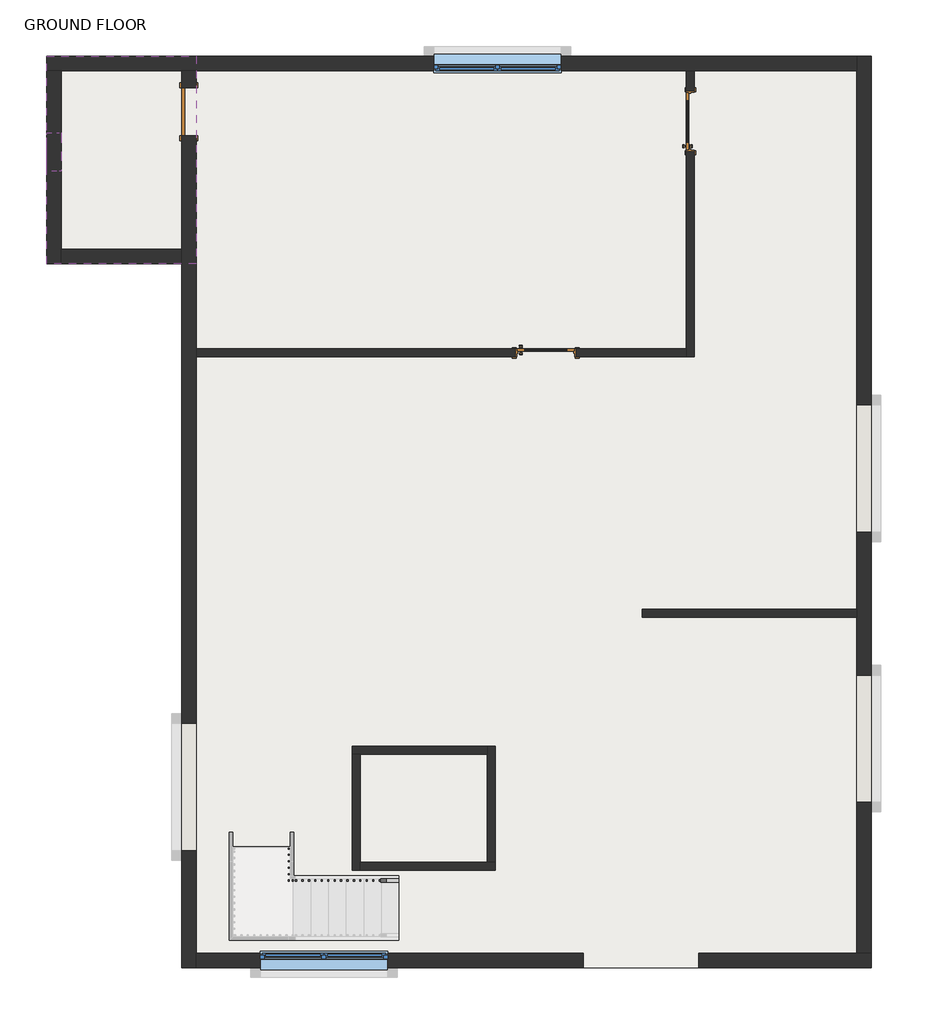
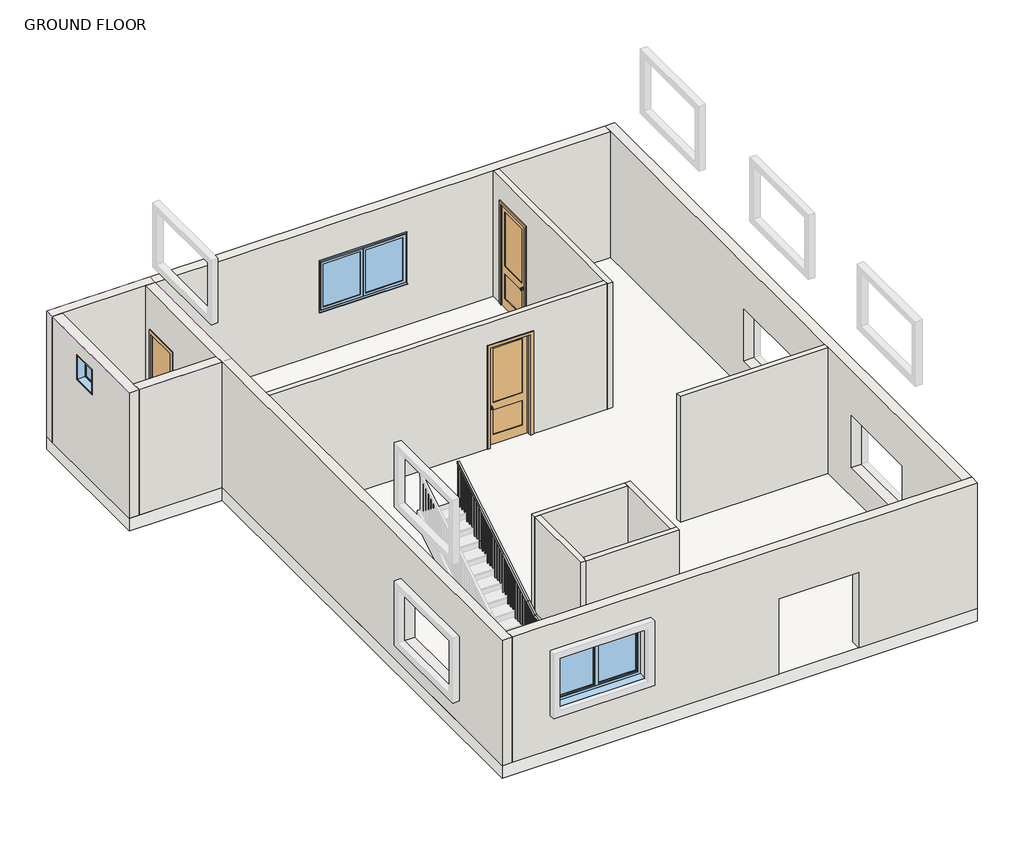
# One storey, part 1 of 2: 13 walls, 3 doors, 3 windows, 1 railing, 1 roof, 1 slab.
"""IFC4 building model written with IfcOpenShell, lengths in millimetres."""

from ifc_helpers import new_model, si_unit, frame, origin, origin_with_axes, place, context, project, spatial, polyline, outline, extrude, faceted_brep, transform, mapped, element, save
from components import door_1a517266, door_a1484949, window_80340324, w2_w2_7b90d420

model = new_model("IFC4")

# Units and contexts
model_context = context("Model", 3, world=origin())
ifc_project = project(units=[si_unit("LENGTHUNIT", "METRE", prefix="MILLI")], contexts=[model_context])

# Site, building, storey
site = spatial("IfcSite", under=ifc_project)
building = spatial("IfcBuilding", under=site)
storey = spatial("IfcBuildingStorey", under=building, Name="GROUND FLOOR", Elevation=304.8)

# Doors
placement = place(None, origin())
door_shape = door_1a517266(model_context)
element("IfcDoor", 1, ObjectType="Door-Interior-Single-2_Panel-Wood : 36\" x 96\"", at=placement, inside=storey, context=model_context, shape_type="MappedRepresentation", body=[
    mapped(door_shape, transform((-1003.5474631, 5446.3811648, 304.8), x_axis=(1.0, 0.0, 0.0), y_axis=(0.0, 1.0, 0.0), z_axis=(0.0, 0.0, 1.0))),
])
element("IfcDoor", 2, ObjectType="Door-Interior-Single-2_Panel-Wood : 36\" x 96\"", at=placement, inside=storey, context=model_context, shape_type="MappedRepresentation", body=[
    mapped(door_shape, transform((1279.2775369, 9100.8061648, 304.8), x_axis=(0.0, 1.0, 0.0), y_axis=(-1.0, 0.0, 0.0), z_axis=(0.0, 0.0, 1.0))),
])
door_2_shape = door_a1484949(model_context)
element("IfcDoor", 3, ObjectType="Single-Flush : 30\" x 80\"", at=placement, inside=storey, context=model_context, shape_type="MappedRepresentation", body=[
    mapped(door_2_shape, transform((-6642.3474631, 9253.2061648, 304.8), x_axis=(0.0, 1.0, 0.0), y_axis=(-1.0, 0.0, 0.0), z_axis=(0.0, 0.0, 1.0))),
])

# Railing
element("IfcRailing", 4, ObjectType="Handrail - Rectangular", at=placement, inside=storey, context=model_context, shape_type="SolidModel", body=[
    faceted_brep([(-3322.4601025, -2919.857314, 1388.5333333), (-3322.4601025, -2919.857314, 1329.1318731), (-3322.4601025, -2869.057314, 1329.1318731), (-3322.4601025, -2869.057314, 1388.5333333), (-4998.8601025, -2919.857314, 2404.5333333), (-5013.0525119, -2919.857314, 2353.7333333), (-5013.0525119, -2869.057314, 2353.7333333), (-4998.8601025, -2869.057314, 2404.5333333), (-5087.9750936, -2919.857314, 2404.5333333), (-5087.9750936, -2919.857314, 2353.7333333), (-5037.1750936, -2869.057314, 2353.7333333), (-5037.1750936, -2869.057314, 2404.5333333), (-5087.9750936, -2670.5272484, 2404.5333333), (-5087.9750936, -2656.334839, 2353.7333333), (-5037.1750936, -2656.334839, 2353.7333333), (-5037.1750936, -2670.5272484, 2404.5333333), (-5087.9750936, -2391.1272484, 2573.8666667), (-5087.9750936, -2364.7975213, 2530.4226168), (-5037.1750936, -2364.7975213, 2530.4226168), (-5037.1750936, -2391.1272484, 2573.8666667), (-5087.9750936, 402.8727516, 4267.2), (-5037.1750936, 402.8727516, 4267.2), (-5037.1750936, 402.8727516, 4207.7985397), (-5087.9750936, 402.8727516, 4207.7985397)], [[[0, 1, 2, 3]], [[1, 0, 4, 5]], [[2, 1, 5, 6]], [[3, 2, 6, 7]], [[0, 3, 7, 4]], [[5, 4, 8, 9]], [[6, 5, 9, 10]], [[7, 6, 10, 11]], [[4, 7, 11, 8]], [[9, 8, 12, 13]], [[10, 9, 13, 14]], [[11, 10, 14, 15]], [[8, 11, 15, 12]], [[13, 12, 16, 17]], [[14, 13, 17, 18]], [[15, 14, 18, 19]], [[12, 15, 19, 16]], [[20, 21, 22, 23]], [[17, 16, 20, 23]], [[18, 17, 23, 22]], [[19, 18, 22, 21]], [[16, 19, 21, 20]]]),
    extrude(outline(polyline([(342.5477516, 4171.2379337), (361.5977516, 4182.7833882), (361.5977516, 3183.4666667), (342.5477516, 3183.4666667), (342.5477516, 4171.2379337)])), frame((-5072.1000936, 0.0, 0.0), z_axis=(1.0, 0.0, 0.0), x_axis=(0.0, 1.0, 0.0)), (0.0, 0.0, 1.0), 19.05),
    extrude(outline(polyline([(240.9477516, 4109.6621761), (259.9977516, 4121.2076307), (259.9977516, 3183.4666667), (240.9477516, 3183.4666667), (240.9477516, 4109.6621761)])), frame((-5072.1000936, 0.0, 0.0), z_axis=(1.0, 0.0, 0.0), x_axis=(0.0, 1.0, 0.0)), (0.0, 0.0, 1.0), 19.05),
    extrude(outline(polyline([(139.3477516, 4048.0864185), (158.3977516, 4059.6318731), (158.3977516, 3183.4666667), (139.3477516, 3183.4666667), (139.3477516, 4048.0864185)])), frame((-5072.1000936, 0.0, 0.0), z_axis=(1.0, 0.0, 0.0), x_axis=(0.0, 1.0, 0.0)), (0.0, 0.0, 1.0), 19.05),
    extrude(outline(polyline([(37.7477516, 3986.510661), (56.7977516, 3998.0561155), (56.7977516, 3014.1333333), (37.7477516, 3014.1333333), (37.7477516, 3986.510661)])), frame((-5072.1000936, 0.0, 0.0), z_axis=(1.0, 0.0, 0.0), x_axis=(0.0, 1.0, 0.0)), (0.0, 0.0, 1.0), 19.05),
    extrude(outline(polyline([(-63.8522484, 3924.9349034), (-44.8022484, 3936.4803579), (-44.8022484, 3014.1333333), (-63.8522484, 3014.1333333), (-63.8522484, 3924.9349034)])), frame((-5072.1000936, 0.0, 0.0), z_axis=(1.0, 0.0, 0.0), x_axis=(0.0, 1.0, 0.0)), (0.0, 0.0, 1.0), 19.05),
    extrude(outline(polyline([(-165.4522484, 3863.3591458), (-146.4022484, 3874.9046004), (-146.4022484, 3014.1333333), (-165.4522484, 3014.1333333), (-165.4522484, 3863.3591458)])), frame((-5072.1000936, 0.0, 0.0), z_axis=(1.0, 0.0, 0.0), x_axis=(0.0, 1.0, 0.0)), (0.0, 0.0, 1.0), 19.05),
    extrude(outline(polyline([(-267.0522484, 3801.7833882), (-248.0022484, 3813.3288428), (-248.0022484, 2844.8), (-267.0522484, 2844.8), (-267.0522484, 3801.7833882)])), frame((-5072.1000936, 0.0, 0.0), z_axis=(1.0, 0.0, 0.0), x_axis=(0.0, 1.0, 0.0)), (0.0, 0.0, 1.0), 19.05),
    extrude(outline(polyline([(-368.6522484, 3740.2076307), (-349.6022484, 3751.7530852), (-349.6022484, 2844.8), (-368.6522484, 2844.8), (-368.6522484, 3740.2076307)])), frame((-5072.1000936, 0.0, 0.0), z_axis=(1.0, 0.0, 0.0), x_axis=(0.0, 1.0, 0.0)), (0.0, 0.0, 1.0), 19.05),
    extrude(outline(polyline([(-470.2522484, 3678.6318731), (-451.2022484, 3690.1773276), (-451.2022484, 2675.4666667), (-470.2522484, 2675.4666667), (-470.2522484, 3678.6318731)])), frame((-5072.1000936, 0.0, 0.0), z_axis=(1.0, 0.0, 0.0), x_axis=(0.0, 1.0, 0.0)), (0.0, 0.0, 1.0), 19.05),
    extrude(outline(polyline([(-571.8522484, 3617.0561155), (-552.8022484, 3628.60157), (-552.8022484, 2675.4666667), (-571.8522484, 2675.4666667), (-571.8522484, 3617.0561155)])), frame((-5072.1000936, 0.0, 0.0), z_axis=(1.0, 0.0, 0.0), x_axis=(0.0, 1.0, 0.0)), (0.0, 0.0, 1.0), 19.05),
    extrude(outline(polyline([(-673.4522484, 3555.4803579), (-654.4022484, 3567.0258125), (-654.4022484, 2675.4666667), (-673.4522484, 2675.4666667), (-673.4522484, 3555.4803579)])), frame((-5072.1000936, 0.0, 0.0), z_axis=(1.0, 0.0, 0.0), x_axis=(0.0, 1.0, 0.0)), (0.0, 0.0, 1.0), 19.05),
    extrude(outline(polyline([(-775.0522484, 3493.9046004), (-756.0022484, 3505.4500549), (-756.0022484, 2506.1333333), (-775.0522484, 2506.1333333), (-775.0522484, 3493.9046004)])), frame((-5072.1000936, 0.0, 0.0), z_axis=(1.0, 0.0, 0.0), x_axis=(0.0, 1.0, 0.0)), (0.0, 0.0, 1.0), 19.05),
    extrude(outline(polyline([(-876.6522484, 3432.3288428), (-857.6022484, 3443.8742973), (-857.6022484, 2506.1333333), (-876.6522484, 2506.1333333), (-876.6522484, 3432.3288428)])), frame((-5072.1000936, 0.0, 0.0), z_axis=(1.0, 0.0, 0.0), x_axis=(0.0, 1.0, 0.0)), (0.0, 0.0, 1.0), 19.05),
    extrude(outline(polyline([(-978.2522484, 3370.7530852), (-959.2022484, 3382.2985397), (-959.2022484, 2506.1333333), (-978.2522484, 2506.1333333), (-978.2522484, 3370.7530852)])), frame((-5072.1000936, 0.0, 0.0), z_axis=(1.0, 0.0, 0.0), x_axis=(0.0, 1.0, 0.0)), (0.0, 0.0, 1.0), 19.05),
    extrude(outline(polyline([(-1079.8522484, 3309.1773276), (-1060.8022484, 3320.7227822), (-1060.8022484, 2336.8), (-1079.8522484, 2336.8), (-1079.8522484, 3309.1773276)])), frame((-5072.1000936, 0.0, 0.0), z_axis=(1.0, 0.0, 0.0), x_axis=(0.0, 1.0, 0.0)), (0.0, 0.0, 1.0), 19.05),
    extrude(outline(polyline([(-1181.4522484, 3247.60157), (-1162.4022484, 3259.1470246), (-1162.4022484, 2336.8), (-1181.4522484, 2336.8), (-1181.4522484, 3247.60157)])), frame((-5072.1000936, 0.0, 0.0), z_axis=(1.0, 0.0, 0.0), x_axis=(0.0, 1.0, 0.0)), (0.0, 0.0, 1.0), 19.05),
    extrude(outline(polyline([(-1283.0522484, 3186.0258125), (-1264.0022484, 3197.571267), (-1264.0022484, 2336.8), (-1283.0522484, 2336.8), (-1283.0522484, 3186.0258125)])), frame((-5072.1000936, 0.0, 0.0), z_axis=(1.0, 0.0, 0.0), x_axis=(0.0, 1.0, 0.0)), (0.0, 0.0, 1.0), 19.05),
    extrude(outline(polyline([(-1384.6522484, 3124.4500549), (-1365.6022484, 3135.9955094), (-1365.6022484, 2167.4666667), (-1384.6522484, 2167.4666667), (-1384.6522484, 3124.4500549)])), frame((-5072.1000936, 0.0, 0.0), z_axis=(1.0, 0.0, 0.0), x_axis=(0.0, 1.0, 0.0)), (0.0, 0.0, 1.0), 19.05),
    extrude(outline(polyline([(-1486.2522484, 3062.8742973), (-1467.2022484, 3074.4197519), (-1467.2022484, 2167.4666667), (-1486.2522484, 2167.4666667), (-1486.2522484, 3062.8742973)])), frame((-5072.1000936, 0.0, 0.0), z_axis=(1.0, 0.0, 0.0), x_axis=(0.0, 1.0, 0.0)), (0.0, 0.0, 1.0), 19.05),
    extrude(outline(polyline([(-1587.8522484, 3001.2985397), (-1568.8022484, 3012.8439943), (-1568.8022484, 1998.1333333), (-1587.8522484, 1998.1333333), (-1587.8522484, 3001.2985397)])), frame((-5072.1000936, 0.0, 0.0), z_axis=(1.0, 0.0, 0.0), x_axis=(0.0, 1.0, 0.0)), (0.0, 0.0, 1.0), 19.05),
    extrude(outline(polyline([(-1689.4522484, 2939.7227822), (-1670.4022484, 2951.2682367), (-1670.4022484, 1998.1333333), (-1689.4522484, 1998.1333333), (-1689.4522484, 2939.7227822)])), frame((-5072.1000936, 0.0, 0.0), z_axis=(1.0, 0.0, 0.0), x_axis=(0.0, 1.0, 0.0)), (0.0, 0.0, 1.0), 19.05),
    extrude(outline(polyline([(-1791.0522484, 2878.1470246), (-1772.0022484, 2889.6924791), (-1772.0022484, 1998.1333333), (-1791.0522484, 1998.1333333), (-1791.0522484, 2878.1470246)])), frame((-5072.1000936, 0.0, 0.0), z_axis=(1.0, 0.0, 0.0), x_axis=(0.0, 1.0, 0.0)), (0.0, 0.0, 1.0), 19.05),
    extrude(outline(polyline([(-1892.6522484, 2816.571267), (-1873.6022484, 2828.1167216), (-1873.6022484, 1828.8), (-1892.6522484, 1828.8), (-1892.6522484, 2816.571267)])), frame((-5072.1000936, 0.0, 0.0), z_axis=(1.0, 0.0, 0.0), x_axis=(0.0, 1.0, 0.0)), (0.0, 0.0, 1.0), 19.05),
    extrude(outline(polyline([(-1994.2522484, 2754.9955094), (-1975.2022484, 2766.540964), (-1975.2022484, 1828.8), (-1994.2522484, 1828.8), (-1994.2522484, 2754.9955094)])), frame((-5072.1000936, 0.0, 0.0), z_axis=(1.0, 0.0, 0.0), x_axis=(0.0, 1.0, 0.0)), (0.0, 0.0, 1.0), 19.05),
    extrude(outline(polyline([(-2095.8522484, 2693.4197519), (-2076.8022484, 2704.9652064), (-2076.8022484, 1828.8), (-2095.8522484, 1828.8), (-2095.8522484, 2693.4197519)])), frame((-5072.1000936, 0.0, 0.0), z_axis=(1.0, 0.0, 0.0), x_axis=(0.0, 1.0, 0.0)), (0.0, 0.0, 1.0), 19.05),
    extrude(outline(polyline([(-2197.4522484, 2631.8439943), (-2178.4022484, 2643.3894488), (-2178.4022484, 1659.4666667), (-2197.4522484, 1659.4666667), (-2197.4522484, 2631.8439943)])), frame((-5072.1000936, 0.0, 0.0), z_axis=(1.0, 0.0, 0.0), x_axis=(0.0, 1.0, 0.0)), (0.0, 0.0, 1.0), 19.05),
    extrude(outline(polyline([(-2299.0522484, 2570.2682367), (-2280.0022484, 2581.8136913), (-2280.0022484, 1659.4666667), (-2299.0522484, 1659.4666667), (-2299.0522484, 2570.2682367)])), frame((-5072.1000936, 0.0, 0.0), z_axis=(1.0, 0.0, 0.0), x_axis=(0.0, 1.0, 0.0)), (0.0, 0.0, 1.0), 19.05),
    extrude(outline(polyline([(-2497.582314, 2449.9469848), (-2478.532314, 2461.4924394), (-2478.532314, 1490.1333333), (-2497.582314, 1490.1333333), (-2497.582314, 2449.9469848)])), frame((-5072.1000936, 0.0, 0.0), z_axis=(1.0, 0.0, 0.0), x_axis=(0.0, 1.0, 0.0)), (0.0, 0.0, 1.0), 19.05),
    extrude(outline(polyline([(-2599.182314, 2388.3712273), (-2580.132314, 2399.9166818), (-2580.132314, 1490.1333333), (-2599.182314, 1490.1333333), (-2599.182314, 2388.3712273)])), frame((-5072.1000936, 0.0, 0.0), z_axis=(1.0, 0.0, 0.0), x_axis=(0.0, 1.0, 0.0)), (0.0, 0.0, 1.0), 19.05),
    extrude(outline(polyline([(-5053.0500936, -2700.782314), (-5072.1000936, -2700.782314), (-5072.1000936, -2681.732314), (-5053.0500936, -2681.732314), (-5053.0500936, -2700.782314)])), frame((0.0, 0.0, 1490.1333333), z_axis=(0.0, 0.0, 1.0), x_axis=(1.0, 0.0, 0.0)), (0.0, 0.0, 1.0), 863.6),
    extrude(outline(polyline([(-5053.0500936, -2802.382314), (-5072.1000936, -2802.382314), (-5072.1000936, -2783.332314), (-5053.0500936, -2783.332314), (-5053.0500936, -2802.382314)])), frame((0.0, 0.0, 1490.1333333), z_axis=(0.0, 0.0, 1.0), x_axis=(1.0, 0.0, 0.0)), (0.0, 0.0, 1.0), 863.6),
    extrude(outline(polyline([(2308.571267, -4938.5351025), (2320.1167216, -4957.5851025), (1320.8, -4957.5851025), (1320.8, -4938.5351025), (2308.571267, -4938.5351025)])), frame((0.0, -2903.982314, 0.0), z_axis=(0.0, 1.0, 0.0), x_axis=(0.0, 0.0, 1.0)), (0.0, 0.0, 1.0), 19.05),
    extrude(outline(polyline([(2246.9955094, -4836.9351025), (2258.540964, -4855.9851025), (1320.8, -4855.9851025), (1320.8, -4836.9351025), (2246.9955094, -4836.9351025)])), frame((0.0, -2903.982314, 0.0), z_axis=(0.0, 1.0, 0.0), x_axis=(0.0, 0.0, 1.0)), (0.0, 0.0, 1.0), 19.05),
    extrude(outline(polyline([(2185.4197519, -4735.3351025), (2196.9652064, -4754.3851025), (1320.8, -4754.3851025), (1320.8, -4735.3351025), (2185.4197519, -4735.3351025)])), frame((0.0, -2903.982314, 0.0), z_axis=(0.0, 1.0, 0.0), x_axis=(0.0, 0.0, 1.0)), (0.0, 0.0, 1.0), 19.05),
    extrude(outline(polyline([(2123.8439943, -4633.7351025), (2135.3894488, -4652.7851025), (1151.4666667, -4652.7851025), (1151.4666667, -4633.7351025), (2123.8439943, -4633.7351025)])), frame((0.0, -2903.982314, 0.0), z_axis=(0.0, 1.0, 0.0), x_axis=(0.0, 0.0, 1.0)), (0.0, 0.0, 1.0), 19.05),
    extrude(outline(polyline([(2062.2682367, -4532.1351025), (2073.8136913, -4551.1851025), (1151.4666667, -4551.1851025), (1151.4666667, -4532.1351025), (2062.2682367, -4532.1351025)])), frame((0.0, -2903.982314, 0.0), z_axis=(0.0, 1.0, 0.0), x_axis=(0.0, 0.0, 1.0)), (0.0, 0.0, 1.0), 19.05),
    extrude(outline(polyline([(2000.6924791, -4430.5351025), (2012.2379337, -4449.5851025), (1151.4666667, -4449.5851025), (1151.4666667, -4430.5351025), (2000.6924791, -4430.5351025)])), frame((0.0, -2903.982314, 0.0), z_axis=(0.0, 1.0, 0.0), x_axis=(0.0, 0.0, 1.0)), (0.0, 0.0, 1.0), 19.05),
    extrude(outline(polyline([(1939.1167216, -4328.9351025), (1950.6621761, -4347.9851025), (982.1333333, -4347.9851025), (982.1333333, -4328.9351025), (1939.1167216, -4328.9351025)])), frame((0.0, -2903.982314, 0.0), z_axis=(0.0, 1.0, 0.0), x_axis=(0.0, 0.0, 1.0)), (0.0, 0.0, 1.0), 19.05),
    extrude(outline(polyline([(1877.540964, -4227.3351025), (1889.0864185, -4246.3851025), (982.1333333, -4246.3851025), (982.1333333, -4227.3351025), (1877.540964, -4227.3351025)])), frame((0.0, -2903.982314, 0.0), z_axis=(0.0, 1.0, 0.0), x_axis=(0.0, 0.0, 1.0)), (0.0, 0.0, 1.0), 19.05),
    extrude(outline(polyline([(1815.9652064, -4125.7351025), (1827.510661, -4144.7851025), (812.8, -4144.7851025), (812.8, -4125.7351025), (1815.9652064, -4125.7351025)])), frame((0.0, -2903.982314, 0.0), z_axis=(0.0, 1.0, 0.0), x_axis=(0.0, 0.0, 1.0)), (0.0, 0.0, 1.0), 19.05),
    extrude(outline(polyline([(1754.3894488, -4024.1351025), (1765.9349034, -4043.1851025), (812.8, -4043.1851025), (812.8, -4024.1351025), (1754.3894488, -4024.1351025)])), frame((0.0, -2903.982314, 0.0), z_axis=(0.0, 1.0, 0.0), x_axis=(0.0, 0.0, 1.0)), (0.0, 0.0, 1.0), 19.05),
    extrude(outline(polyline([(1692.8136913, -3922.5351025), (1704.3591458, -3941.5851025), (812.8, -3941.5851025), (812.8, -3922.5351025), (1692.8136913, -3922.5351025)])), frame((0.0, -2903.982314, 0.0), z_axis=(0.0, 1.0, 0.0), x_axis=(0.0, 0.0, 1.0)), (0.0, 0.0, 1.0), 19.05),
    extrude(outline(polyline([(1631.2379337, -3820.9351025), (1642.7833882, -3839.9851025), (643.4666667, -3839.9851025), (643.4666667, -3820.9351025), (1631.2379337, -3820.9351025)])), frame((0.0, -2903.982314, 0.0), z_axis=(0.0, 1.0, 0.0), x_axis=(0.0, 0.0, 1.0)), (0.0, 0.0, 1.0), 19.05),
    extrude(outline(polyline([(1569.6621761, -3719.3351025), (1581.2076307, -3738.3851025), (643.4666667, -3738.3851025), (643.4666667, -3719.3351025), (1569.6621761, -3719.3351025)])), frame((0.0, -2903.982314, 0.0), z_axis=(0.0, 1.0, 0.0), x_axis=(0.0, 0.0, 1.0)), (0.0, 0.0, 1.0), 19.05),
    extrude(outline(polyline([(1508.0864185, -3617.7351025), (1519.6318731, -3636.7851025), (643.4666667, -3636.7851025), (643.4666667, -3617.7351025), (1508.0864185, -3617.7351025)])), frame((0.0, -2903.982314, 0.0), z_axis=(0.0, 1.0, 0.0), x_axis=(0.0, 0.0, 1.0)), (0.0, 0.0, 1.0), 19.05),
    extrude(outline(polyline([(1446.510661, -3516.1351025), (1458.0561155, -3535.1851025), (474.1333333, -3535.1851025), (474.1333333, -3516.1351025), (1446.510661, -3516.1351025)])), frame((0.0, -2903.982314, 0.0), z_axis=(0.0, 1.0, 0.0), x_axis=(0.0, 0.0, 1.0)), (0.0, 0.0, 1.0), 19.05),
    extrude(outline(polyline([(1384.9349034, -3414.5351025), (1396.4803579, -3433.5851025), (474.1333333, -3433.5851025), (474.1333333, -3414.5351025), (1384.9349034, -3414.5351025)])), frame((0.0, -2903.982314, 0.0), z_axis=(0.0, 1.0, 0.0), x_axis=(0.0, 0.0, 1.0)), (0.0, 0.0, 1.0), 19.05),
    extrude(outline(polyline([(-2400.6522484, 2508.6924791), (-2381.6022484, 2520.2379337), (-2381.6022484, 1490.1333333), (-2400.6522484, 1490.1333333), (-2400.6522484, 2508.6924791)])), frame((-5072.1000936, 0.0, 0.0), z_axis=(1.0, 0.0, 0.0), x_axis=(0.0, 1.0, 0.0)), (0.0, 0.0, 1.0), 19.05),
    extrude(outline(polyline([(-5053.0500936, -2884.932314), (-5053.0500936, -2903.982314), (-5072.1000936, -2903.982314), (-5072.1000936, -2884.932314), (-5053.0500936, -2884.932314)])), frame((0.0, 0.0, 1490.1333333), z_axis=(0.0, 0.0, 1.0), x_axis=(1.0, 0.0, 0.0)), (0.0, 0.0, 1.0), 863.6),
    extrude(outline(polyline([(2339.3591458, -4989.3351025), (2350.9046004, -5008.3851025), (1490.1333333, -5008.3851025), (1490.1333333, -4989.3351025), (2339.3591458, -4989.3351025)])), frame((0.0, -2903.982314, 0.0), z_axis=(0.0, 1.0, 0.0), x_axis=(0.0, 0.0, 1.0)), (0.0, 0.0, 1.0), 19.05),
    extrude(outline(polyline([(383.8227516, 4196.2530852), (402.8727516, 4207.7985397), (402.8727516, 3183.4666667), (383.8227516, 3183.4666667), (383.8227516, 4196.2530852)])), frame((-5072.1000936, 0.0, 0.0), z_axis=(1.0, 0.0, 0.0), x_axis=(0.0, 1.0, 0.0)), (0.0, 0.0, 1.0), 19.05),
    extrude(outline(polyline([(1329.1318731, -3322.4601025), (1340.6773276, -3341.5101025), (474.1333333, -3341.5101025), (474.1333333, -3322.4601025), (1329.1318731, -3322.4601025)])), frame((0.0, -2903.982314, 0.0), z_axis=(0.0, 1.0, 0.0), x_axis=(0.0, 0.0, 1.0)), (0.0, 0.0, 1.0), 19.05),
])

# Roof
element("IfcRoof", 5, ObjectType="ROOFING 6\"", at=placement, inside=storey, context=model_context, shape_type="Brep", body=[
    faceted_brep([(-6528.0474631, 10129.5061648, 3352.8), (-7709.1474631, 8948.4061648, 4238.625), (-8890.2474631, 10129.5061648, 3352.8), (-7709.1474631, 8034.0061648, 4238.625), (-8890.2474631, 6852.9061648, 3352.8), (-6528.0474631, 6852.9061648, 3352.8), (-6528.0474631, 10129.5061648, 3733.8), (-8890.2474631, 10129.5061648, 3733.8), (-7709.1474631, 8948.4061648, 4619.625), (-8890.2474631, 6852.9061648, 3733.8), (-7709.1474631, 8034.0061648, 4619.625), (-6528.0474631, 6852.9061648, 3733.8)], [[[0, 1, 2]], [[2, 1, 3, 4]], [[4, 3, 5]], [[1, 0, 5, 3]], [[6, 7, 8]], [[7, 9, 10, 8]], [[9, 11, 10]], [[6, 8, 10, 11]], [[2, 7, 6, 0]], [[4, 9, 7, 2]], [[5, 11, 9, 4]], [[0, 6, 11, 5]]]),
])

# Slab
element("IfcSlab", 6, ObjectType="MARBLE FLOORING 1'", at=placement, inside=storey, context=model_context, shape_type="SweptSolid", body=[
    extrude(outline(polyline([(4139.9525369, 10129.5061648), (4139.9525369, -4272.2938352), (-6756.6474631, -4272.2938352), (-6756.6474631, 6852.9061648), (-8890.2474631, 6852.9061648), (-8890.2474631, 10129.5061648), (4139.9525369, 10129.5061648)])), origin_with_axes(), (0.0, 0.0, 1.0), 304.8),
])

# Walls
element("IfcWall", 7, ObjectType="EXTERIOR WALL 9\"", at=placement, inside=storey, context=model_context, shape_type="Brep", body=[
    faceted_brep([(-6756.6474631, 9900.9061648, 304.8), (-6756.6474631, 9634.2061648, 304.8), (-6756.6474631, 9634.2061648, 2336.8), (-6756.6474631, 8872.2061648, 2336.8), (-6756.6474631, 8872.2061648, 304.8), (-6756.6474631, 7081.5061648, 304.8), (-6756.6474631, 6852.9061648, 304.8), (-6756.6474631, -4272.2938352, 304.8), (-6756.6474631, -4272.2938352, 3352.8), (-6756.6474631, 6852.9061648, 3352.8), (-6756.6474631, 7081.5061648, 3352.8), (-6756.6474631, 9900.9061648, 3352.8), (-6756.6474631, -409.7938352, 1000.0), (-6756.6474631, -409.7938352, 2260.0), (-6756.6474631, -2419.7938352, 2260.0), (-6756.6474631, -2419.7938352, 1000.0), (-6528.0474631, 9634.2061648, 2336.8), (-6528.0474631, 9634.2061648, 304.8), (-6528.0474631, 9900.9061648, 304.8), (-6528.0474631, 9900.9061648, 3352.8), (-6528.0474631, 5506.7061648, 3352.8), (-6528.0474631, 5379.7061648, 3352.8), (-6528.0474631, -4043.6938352, 3352.8), (-6528.0474631, -4272.2938352, 3352.8), (-6528.0474631, -4272.2938352, 304.8), (-6528.0474631, -4043.6938352, 304.8), (-6528.0474631, 5379.7061648, 304.8), (-6528.0474631, 5506.7061648, 304.8), (-6528.0474631, 8872.2061648, 304.8), (-6528.0474631, 8872.2061648, 2336.8), (-6528.0474631, -409.7938352, 1000.0), (-6528.0474631, -2419.7938352, 1000.0), (-6528.0474631, -2419.7938352, 2260.0), (-6528.0474631, -409.7938352, 2260.0)], [[[0, 1, 2, 3, 4, 5, 6, 7, 8, 9, 10, 11], [12, 13, 14, 15]], [[16, 17, 18, 19, 20, 21, 22, 23, 24, 25, 26, 27, 28, 29], [30, 31, 32, 33]], [[18, 17, 1, 0]], [[28, 27, 26, 25, 24, 7, 6, 5, 4]], [[11, 10, 9, 8, 23, 22, 21, 20, 19]], [[8, 7, 24, 23]], [[0, 11, 19, 18]], [[13, 12, 30, 33]], [[14, 13, 33, 32]], [[15, 14, 32, 31]], [[12, 15, 31, 30]], [[2, 1, 17, 16]], [[3, 2, 16, 29]], [[4, 3, 29, 28]]]),
])
element("IfcWall", 8, ObjectType="EXTERIOR WALL 9\"", at=placement, inside=storey, context=model_context, shape_type="Brep", body=[
    faceted_brep([(4139.9525369, -4272.2938352, 3352.8), (-6528.0474631, -4272.2938352, 3352.8), (-6528.0474631, -4272.2938352, 304.8), (-412.2702791, -4272.2938352, 304.8), (-412.2702791, -4272.2938352, 2133.6), (1416.5297209, -4272.2938352, 2133.6), (1416.5297209, -4272.2938352, 304.8), (4139.9525369, -4272.2938352, 304.8), (-3503.7474631, -4272.2938352, 1304.8), (-5513.7474631, -4272.2938352, 1304.8), (-5513.7474631, -4272.2938352, 2564.8), (-3503.7474631, -4272.2938352, 2564.8), (-6528.0474631, -4043.6938352, 3352.8), (3911.3525369, -4043.6938352, 3352.8), (4139.9525369, -4043.6938352, 3352.8), (4139.9525369, -4043.6938352, 304.8), (3911.3525369, -4043.6938352, 304.8), (1416.5297209, -4043.6938352, 304.8), (1416.5297209, -4043.6938352, 2133.6), (-412.2702791, -4043.6938352, 2133.6), (-412.2702791, -4043.6938352, 304.8), (-6528.0474631, -4043.6938352, 304.8), (-3503.7474631, -4043.6938352, 1304.8), (-3503.7474631, -4043.6938352, 2564.8), (-5513.7474631, -4043.6938352, 2564.8), (-5513.7474631, -4043.6938352, 1304.8)], [[[0, 1, 2, 3, 4, 5, 6, 7], [8, 9, 10, 11]], [[12, 13, 14, 15, 16, 17, 18, 19, 20, 21], [22, 23, 24, 25]], [[2, 21, 20, 3]], [[15, 7, 6, 17, 16]], [[1, 0, 14, 13, 12]], [[2, 1, 12, 21]], [[0, 7, 15, 14]], [[5, 18, 17, 6]], [[19, 4, 3, 20]], [[18, 5, 4, 19]], [[23, 22, 8, 11]], [[24, 23, 11, 10]], [[25, 24, 10, 9]], [[22, 25, 9, 8]]]),
])
element("IfcWall", 9, ObjectType="EXTERIOR WALL 9\"", at=placement, inside=storey, context=model_context, shape_type="Brep", body=[
    faceted_brep([(4139.9525369, -4043.6938352, 304.8), (4139.9525369, 10129.5061648, 304.8), (4139.9525369, 10129.5061648, 3352.8), (4139.9525369, -4043.6938352, 3352.8), (4139.9525369, 352.2061648, 1000.0), (4139.9525369, -1657.7938352, 1000.0), (4139.9525369, -1657.7938352, 2260.0), (4139.9525369, 352.2061648, 2260.0), (4139.9525369, 4619.4061648, 1000.0), (4139.9525369, 2609.4061648, 1000.0), (4139.9525369, 2609.4061648, 2260.0), (4139.9525369, 4619.4061648, 2260.0), (3911.3525369, -4043.6938352, 304.8), (3911.3525369, -4043.6938352, 3352.8), (3911.3525369, 1264.9061648, 3352.8), (3911.3525369, 1391.9061648, 3352.8), (3911.3525369, 6446.5061648, 3352.8), (3911.3525369, 6573.5061648, 3352.8), (3911.3525369, 9900.9061648, 3352.8), (3911.3525369, 10129.5061648, 3352.8), (3911.3525369, 10129.5061648, 304.8), (3911.3525369, 9900.9061648, 304.8), (3911.3525369, 6573.5061648, 304.8), (3911.3525369, 6446.5061648, 304.8), (3911.3525369, 1391.9061648, 304.8), (3911.3525369, 1264.9061648, 304.8), (3911.3525369, 352.2061648, 1000.0), (3911.3525369, 352.2061648, 2260.0), (3911.3525369, -1657.7938352, 2260.0), (3911.3525369, -1657.7938352, 1000.0), (3911.3525369, 4619.4061648, 1000.0), (3911.3525369, 4619.4061648, 2260.0), (3911.3525369, 2609.4061648, 2260.0), (3911.3525369, 2609.4061648, 1000.0)], [[[0, 1, 2, 3], [4, 5, 6, 7], [8, 9, 10, 11]], [[12, 13, 14, 15, 16, 17, 18, 19, 20, 21, 22, 23, 24, 25], [26, 27, 28, 29], [30, 31, 32, 33]], [[1, 0, 12, 25, 24, 23, 22, 21, 20]], [[3, 2, 19, 18, 17, 16, 15, 14, 13]], [[0, 3, 13, 12]], [[2, 1, 20, 19]], [[27, 26, 4, 7]], [[28, 27, 7, 6]], [[29, 28, 6, 5]], [[26, 29, 5, 4]], [[31, 30, 8, 11]], [[32, 31, 11, 10]], [[33, 32, 10, 9]], [[30, 33, 9, 8]]]),
])
element("IfcWall", 10, ObjectType="EXTERIOR WALL 9\"", at=placement, inside=storey, context=model_context, shape_type="Brep", body=[
    faceted_brep([(3911.3525369, 10129.5061648, 304.8), (-8890.2474631, 10129.5061648, 304.8), (-8890.2474631, 10129.5061648, 3352.8), (3911.3525369, 10129.5061648, 3352.8), (-2770.5474631, 10129.5061648, 1304.8), (-760.5474631, 10129.5061648, 1304.8), (-760.5474631, 10129.5061648, 2564.8), (-2770.5474631, 10129.5061648, 2564.8), (3911.3525369, 9900.9061648, 304.8), (3911.3525369, 9900.9061648, 3352.8), (1345.9525369, 9900.9061648, 3352.8), (1218.9525369, 9900.9061648, 3352.8), (-6528.0474631, 9900.9061648, 3352.8), (-6756.6474631, 9900.9061648, 3352.8), (-8661.6474631, 9900.9061648, 3352.8), (-8890.2474631, 9900.9061648, 3352.8), (-8890.2474631, 9900.9061648, 304.8), (-8661.6474631, 9900.9061648, 304.8), (-6756.6474631, 9900.9061648, 304.8), (-6528.0474631, 9900.9061648, 304.8), (1218.9525369, 9900.9061648, 304.8), (1345.9525369, 9900.9061648, 304.8), (-2770.5474631, 9900.9061648, 1304.8), (-2770.5474631, 9900.9061648, 2564.8), (-760.5474631, 9900.9061648, 2564.8), (-760.5474631, 9900.9061648, 1304.8)], [[[0, 1, 2, 3], [4, 5, 6, 7]], [[8, 9, 10, 11, 12, 13, 14, 15, 16, 17, 18, 19, 20, 21], [22, 23, 24, 25]], [[1, 0, 8, 21, 20, 19, 18, 17, 16]], [[3, 2, 15, 14, 13, 12, 11, 10, 9]], [[0, 3, 9, 8]], [[2, 1, 16, 15]], [[23, 22, 4, 7]], [[24, 23, 7, 6]], [[25, 24, 6, 5]], [[22, 25, 5, 4]]]),
])
element("IfcWall", 11, ObjectType="EXTERIOR WALL 9\"", at=placement, inside=storey, context=model_context, shape_type="Brep", body=[
    faceted_brep([(-8890.2474631, 9900.9061648, 304.8), (-8890.2474631, 6852.9061648, 304.8), (-8890.2474631, 6852.9061648, 3352.8), (-8890.2474631, 9900.9061648, 3352.8), (-8890.2474631, 8313.4061648, 3028.2449085), (-8890.2474631, 8313.4061648, 2418.6449085), (-8890.2474631, 8923.0061648, 2418.6449085), (-8890.2474631, 8923.0061648, 3028.2449085), (-8661.6474631, 9900.9061648, 304.8), (-8661.6474631, 9900.9061648, 3352.8), (-8661.6474631, 7081.5061648, 3352.8), (-8661.6474631, 6852.9061648, 3352.8), (-8661.6474631, 6852.9061648, 304.8), (-8661.6474631, 7081.5061648, 304.8), (-8661.6474631, 8313.4061648, 3028.2449085), (-8661.6474631, 8923.0061648, 3028.2449085), (-8661.6474631, 8923.0061648, 2418.6449085), (-8661.6474631, 8313.4061648, 2418.6449085)], [[[0, 1, 2, 3], [4, 5, 6, 7]], [[8, 9, 10, 11, 12, 13], [14, 15, 16, 17]], [[1, 0, 8, 13, 12]], [[3, 2, 11, 10, 9]], [[0, 3, 9, 8]], [[2, 1, 12, 11]], [[5, 4, 14, 17]], [[6, 5, 17, 16]], [[7, 6, 16, 15]], [[4, 7, 15, 14]]]),
])
element("IfcWall", 12, ObjectType="EXTERIOR WALL 9\"", at=placement, inside=storey, context=model_context, shape_type="SweptSolid", body=[
    extrude(outline(polyline([(-6756.6474631, 6852.9061648), (-8661.6474631, 6852.9061648), (-8661.6474631, 7081.5061648), (-6756.6474631, 7081.5061648), (-6756.6474631, 6852.9061648)])), frame((0.0, 0.0, 304.8), z_axis=(0.0, 0.0, 1.0), x_axis=(1.0, 0.0, 0.0)), (0.0, 0.0, 1.0), 3048.0),
])
element("IfcWall", 13, ObjectType="INTERIOR WALL 5\"", at=placement, inside=storey, context=model_context, shape_type="SweptSolid", body=[
    extrude(outline(polyline([(3352.8, 1218.9525369), (3352.8, -6528.0474631), (304.8, -6528.0474631), (304.8, -1486.1474631), (2768.6, -1486.1474631), (2768.6, -520.9474631), (304.8, -520.9474631), (304.8, 1218.9525369), (3352.8, 1218.9525369)])), frame((0.0, 5379.7061648, 0.0), z_axis=(0.0, 1.0, 0.0), x_axis=(0.0, 0.0, 1.0)), (0.0, 0.0, 1.0), 127.0),
])
element("IfcWall", 14, ObjectType="INTERIOR WALL 5\"", at=placement, inside=storey, context=model_context, shape_type="Brep", body=[
    faceted_brep([(1218.9525369, 5379.7061648, 3352.8), (1218.9525369, 5506.7061648, 3352.8), (1218.9525369, 9900.9061648, 3352.8), (1218.9525369, 9900.9061648, 304.8), (1218.9525369, 9583.4061648, 304.8), (1218.9525369, 9583.4061648, 2768.6), (1218.9525369, 8618.2061648, 2768.6), (1218.9525369, 8618.2061648, 304.8), (1218.9525369, 5506.7061648, 304.8), (1218.9525369, 5379.7061648, 304.8), (1345.9525369, 9900.9061648, 3352.8), (1345.9525369, 6573.5061648, 3352.8), (1345.9525369, 6446.5061648, 3352.8), (1345.9525369, 5379.7061648, 3352.8), (1345.9525369, 5379.7061648, 304.8), (1345.9525369, 6446.5061648, 304.8), (1345.9525369, 6573.5061648, 304.8), (1345.9525369, 8618.2061648, 304.8), (1345.9525369, 8618.2061648, 2768.6), (1345.9525369, 9583.4061648, 2768.6), (1345.9525369, 9583.4061648, 304.8), (1345.9525369, 9900.9061648, 304.8)], [[[0, 1, 2, 3, 4, 5, 6, 7, 8, 9]], [[10, 11, 12, 13, 14, 15, 16, 17, 18, 19, 20, 21]], [[3, 21, 20, 4]], [[14, 9, 8, 7, 17, 16, 15]], [[2, 1, 0, 13, 12, 11, 10]], [[3, 2, 10, 21]], [[0, 9, 14, 13]], [[19, 5, 4, 20]], [[5, 19, 18, 6]], [[6, 18, 17, 7]]]),
])
element("IfcWall", 15, ObjectType="INTERIOR WALL 5\"", at=placement, inside=storey, context=model_context, shape_type="SweptSolid", body=[
    extrude(outline(polyline([(520.4525369, 1391.9061648), (3911.3525369, 1391.9061648), (3911.3525369, 1264.9061648), (520.4525369, 1264.9061648), (520.4525369, 1391.9061648)])), frame((0.0, 0.0, 304.8), z_axis=(0.0, 0.0, 1.0), x_axis=(1.0, 0.0, 0.0)), (0.0, 0.0, 1.0), 3048.0),
])
element("IfcWall", 16, ObjectType="INTERIOR WALL 5\"", at=placement, inside=storey, context=model_context, shape_type="Brep", body=[
    faceted_brep([(-4062.7930952, -899.3791472, 304.8), (-3935.7930952, -899.3791472, 304.8), (-1929.1930952, -899.3791472, 304.8), (-1929.1930952, -899.3791472, 3352.8), (-3935.7930952, -899.3791472, 3352.8), (-4062.7930952, -899.3791472, 3352.8), (-4062.7930952, -772.3791472, 304.8), (-4062.7930952, -772.3791472, 3352.8), (-1929.1930952, -772.3791472, 3352.8), (-1929.1930952, -772.3791472, 304.8)], [[[0, 1, 2, 3, 4, 5]], [[6, 7, 8, 9]], [[2, 1, 0, 6, 9]], [[5, 4, 3, 8, 7]], [[0, 5, 7, 6]], [[3, 2, 9, 8]]]),
])
element("IfcWall", 17, ObjectType="INTERIOR WALL 5\"", at=placement, inside=storey, context=model_context, shape_type="Brep", body=[
    faceted_brep([(-3935.7930952, -2728.1791472, 304.8), (-3935.7930952, -2601.1791472, 304.8), (-3935.7930952, -899.3791472, 304.8), (-3935.7930952, -899.3791472, 3352.8), (-3935.7930952, -2601.1791472, 3352.8), (-3935.7930952, -2728.1791472, 3352.8), (-4062.7930952, -2728.1791472, 304.8), (-4062.7930952, -2728.1791472, 3352.8), (-4062.7930952, -899.3791472, 3352.8), (-4062.7930952, -899.3791472, 304.8)], [[[0, 1, 2, 3, 4, 5]], [[6, 7, 8, 9]], [[2, 1, 0, 6, 9]], [[5, 4, 3, 8, 7]], [[0, 5, 7, 6]], [[3, 2, 9, 8]]]),
])
element("IfcWall", 18, ObjectType="INTERIOR WALL 5\"", at=placement, inside=storey, context=model_context, shape_type="Brep", body=[
    faceted_brep([(-1802.1930952, -2601.1791472, 304.8), (-1929.1930952, -2601.1791472, 304.8), (-3935.7930952, -2601.1791472, 304.8), (-3935.7930952, -2601.1791472, 3352.8), (-1929.1930952, -2601.1791472, 3352.8), (-1802.1930952, -2601.1791472, 3352.8), (-1802.1930952, -2728.1791472, 304.8), (-1802.1930952, -2728.1791472, 3352.8), (-3935.7930952, -2728.1791472, 3352.8), (-3935.7930952, -2728.1791472, 304.8)], [[[0, 1, 2, 3, 4, 5]], [[6, 7, 8, 9]], [[2, 1, 0, 6, 9]], [[5, 4, 3, 8, 7]], [[0, 5, 7, 6]], [[3, 2, 9, 8]]]),
])
element("IfcWall", 19, ObjectType="INTERIOR WALL 5\"", at=placement, inside=storey, context=model_context, shape_type="Brep", body=[
    faceted_brep([(-1929.1930952, -772.3791472, 304.8), (-1929.1930952, -899.3791472, 304.8), (-1929.1930952, -2601.1791472, 304.8), (-1929.1930952, -2601.1791472, 3352.8), (-1929.1930952, -899.3791472, 3352.8), (-1929.1930952, -772.3791472, 3352.8), (-1802.1930952, -772.3791472, 304.8), (-1802.1930952, -772.3791472, 3352.8), (-1802.1930952, -2601.1791472, 3352.8), (-1802.1930952, -2601.1791472, 304.8)], [[[0, 1, 2, 3, 4, 5]], [[6, 7, 8, 9]], [[2, 1, 0, 6, 9]], [[5, 4, 3, 8, 7]], [[0, 5, 7, 6]], [[3, 2, 9, 8]]]),
])

# Windows
window_shape = window_80340324(model_context)
element("IfcWindow", 20, ObjectType="Fixed : 24\" x 24\"", at=placement, inside=storey, context=model_context, shape_type="MappedRepresentation", body=[
    mapped(window_shape, transform((-8775.9474631, 8580.1061648, 1504.2449085), x_axis=(0.0, -1.0, 0.0), y_axis=(1.0, 0.0, 0.0), z_axis=(0.0, 0.0, 1.0))),
])
w2_w2_shape = w2_w2_7b90d420(model_context)
element("IfcWindow", 21, ObjectType="w2 : w2", at=placement, inside=storey, context=model_context, shape_type="MappedRepresentation", body=[
    mapped(w2_w2_shape, transform((-1765.5474631, 10015.2061648, 304.8), x_axis=(1.0, 0.0, 0.0), y_axis=(0.0, 1.0, 0.0), z_axis=(0.0, 0.0, 1.0))),
])
element("IfcWindow", 22, ObjectType="w2 : w2", at=placement, inside=storey, context=model_context, shape_type="MappedRepresentation", body=[
    mapped(w2_w2_shape, transform((-4508.7474631, -4157.9938352, 304.8), x_axis=(-1.0, 0.0, 0.0), y_axis=(0.0, -1.0, 0.0), z_axis=(0.0, 0.0, 1.0))),
])

save(model, "model.ifc")

# Revit data of these elements
# Type "Door-Interior-Single-2_Panel-Wood : 36\" x 96\""
#   Type Mark = "10"
#   Assembly Code = "C1020300"
#   Analytic Construction = "Wooden"
#   Top Rail = 0' - 4 11/16"
#   Thickness = 0' - 1 3/8"
#   Thermal Resistance (R) = 2.5876 (h·ft²·°F)/BTU
#   Swing Angle [instance default] = 90.00°
#   Stiles = 0' - 4 3/4"
#   Rough Width = 3' - 2"
#   Rough Height = 8' - 1"
#   Lock Rail = 0' - 7 1/2"
#   Height = 8' - 0"
#   Width = 3' - 0"
#   Heat Transfer Coefficient (U) = 0.3865 BTU/(h·ft²·°F)
#   Bottom Rail = 0' - 9 1/8"
#   Trim Material = Cherry
#   Panel Material = Cherry
#   Frame Material = Cherry
#   Door Handle Material = Aluminum
#   Visual Light Transmittance = 0
#   Solar Heat Gain Coefficient = 0
#   Wall Closure = (empty or 0)
#   Function = (empty or 0)
# Type "Single-Flush : 30\" x 80\""
#   Type Mark = "5"
#   Construction Type Id = "MDOOR"
#   Assembly Code = "C1020"
#   Analytic Construction = "Metal"
#   Thickness = 0' - 2"
#   Heat Transfer Coefficient (U) = 0.651978 BTU/(h·ft²·°F)
#   Height = 6' - 8"
#   Trim Projection Ext = 0' - 1"
#   Trim Projection Int = 0' - 1"
#   Trim Width = 0' - 3"
#   Width = 2' - 6"
#   Define Thermal Properties by = 1
#   Define Thermal Properties by = 1
#   Door Material = Door - Panel
#   Frame Material = Door - Frame
#   Visual Light Transmittance = 0
#   Solar Heat Gain Coefficient = 0
#   Function = (empty or 0)
#   Wall Closure = (empty or 0)
# Type "Handrail - Rectangular"
#   Assembly Code = "C2010400"
#   built-in parameter 1008612 = 0.0416667 (stored number, unit not read)
#   built-in parameter 1008611 = 0.0416667 (stored number, unit not read)
#   built-in parameter 1008609 = 0.333333 (stored number, unit not read)
#   built-in parameter 1008604 = 0.166667 (stored number, unit not read)
#   built-in parameter 1008603 = 0.166667 (stored number, unit not read)
#   Railing Height = 3' - 0"
#   built-in parameter 1008630 = 2
#   built-in parameter 1008610 = 2
#   built-in parameter 1008618 = Baluster - Square : 3/4"
# Type "ROOFING 6\""
#   Assembly Code = "B1020"
#   Layers, outside or top first: 1' - 0" "ROOFING" (function 1)
# Type "MARBLE FLOORING 1'"
#   Assembly Code = "B1010"
#   Function = 0
#   Layers, outside or top first: 1' - 0" "MARBLE MATERIAL" (function 1)
# Type "EXTERIOR WALL 9\""
#   Assembly Code = "B2010"
#   Layers, outside or top first: 0' - 9" "OFF WHITE COLOUR" (function 1)
# Type "INTERIOR WALL 5\""
#   Assembly Code = "B2010"
#   Layers, outside or top first: 0' - 5" "OFF WHITE COLOUR" (function 1)
# Type "Fixed : 24\" x 24\""
#   Type Mark = "3"
#   Construction Type Id = "GSP4R"
#   Assembly Code = "B2020100"
#   Analytic Construction = "1/8 in Pilkington single glazing"
#   Visual Light Transmittance = 0.9
#   Solar Heat Gain Coefficient = 0.78
#   Heat Transfer Coefficient (U) = 0.6496 BTU/(h·ft²·°F)
#   Height = 2' - 0"
#   Default Sill Height = 3' - 0"
#   Width = 2' - 0"
#   Window Inset = 0' - 0 3/4"
#   Define Thermal Properties by = 1
#   Define Thermal Properties by = 1
#   Glass Pane Material = Glass
#   Sash Material = Sash
#   Wall Closure = (empty or 0)
# Type "w2 : w2"
#   Type Mark = "18"
#   Operation = "DoublePanelVertical"
#   Keynote = "16.05.01"
#   Analytic Construction = "<None>"
#   Rough Width = 6' - 7.13386"
#   Rough Height = 4' - 1.6063"
#   Rahmentiefe = 0' - 2.3622"
#   Rahmenhöhe unten = 0' - 3.14961"
#   Rahmehöhe oben = 0' - 3.14961"
#   Rahmenbreite = 0' - 2.3622"
#   Heat Transfer Coefficient (U) = 2.81836 BTU/(h·ft²·°F)
#   Height = 4' - 1.6063"
#   Flügeltiefe = 0' - 2.3622"
#   Flügelbreite = 0' - 2.3622"
#   Einbautiefe (von außen) [instance default] = 0' - 5.51181"
#   Width = 6' - 7.13386"
#   Kippflügel [instance default] = yes
#   Drehflügel im Grundriß darstellen [instance default] = no
#   Drehflügel [instance default] = yes
#   Define Thermal Properties by = 1
#   Rahmen [instance default] = none
#   Glas [instance default] = blue glass
#   Flügel [instance default] = WINDOW COLOUR WHITE
#   Fensterbank aussen [instance default] = WINDOW COLOUR WHITE
#   Fensterbank innen [instance default] = WINDOW COLOUR WHITE
#   Visual Light Transmittance = 0
#   Thermal Resistance (R) = 0
#   Solar Heat Gain Coefficient = 0
#   Wall Closure = (empty or 0)
# Elements 1, 2 (IfcDoor, "Door-Interior-Single-2_Panel-Wood : 36\" x 96\"")
#   Swing Angle = 90.00°
#   Phase Created = New Construction
#   Materials on its faces: "Cherry", "Aluminum"
# Element 3 (IfcDoor, "Single-Flush : 30\" x 80\"")
#   Phase Created = New Construction
#   Materials on its faces: "Door - Frame", "Door - Panel"
# Element 4 (IfcRailing, "Handrail - Rectangular")
#   Phase Created = New Construction
# Element 5 (IfcRoof, "ROOFING 6\"")
#   built-in parameter 1001705 = 15.1562 (stored number, unit not read)
#   built-in parameter 1001701 = 10 (stored number, unit not read)
#   built-in parameter 1001710 = 33615
#   Phase Created = New Construction
#   Materials on its faces: "ROOFING"
# Element 6 (IfcSlab, "MARBLE FLOORING 1'")
#   Height Offset From Level = 0' - 0"
#   Phase Created = New Construction
#   Materials on its faces: "MARBLE MATERIAL"
# Elements 7, 8, 9, 10, 11, 12 (IfcWall, "EXTERIOR WALL 9\"")
#   Top Offset = 0' - 0"
#   Base Offset = 0' - 0"
#   Unconnected Height = 10' - 0"
#   wall height = 10' - 0"
#   Phase Created = New Construction
#   Base Constraint = GROUND FLOOR
#   Top Constraint = FIRST FLR
#   Materials on its faces: "OFF WHITE COLOUR"
# Elements 13, 14, 15 (IfcWall, "INTERIOR WALL 5\"")
#   Top Offset = 0' - 0"
#   Base Offset = 0' - 0"
#   Unconnected Height = 10' - 0"
#   wall height = 10' - 0"
#   Phase Created = New Construction
#   Base Constraint = GROUND FLOOR
#   Top Constraint = FIRST FLR
#   Materials on its faces: "OFF WHITE COLOUR"
# Elements 16, 17, 18, 19 (IfcWall, "INTERIOR WALL 5\"")
#   Top Offset = 0' - 0"
#   Base Offset = 0' - 0"
#   wall height = 10' - 0"
#   Phase Created = New Construction
#   Base Constraint = GROUND FLOOR
#   Top Constraint = FIRST FLR
#   Materials on its faces: "OFF WHITE COLOUR"
# Element 20 (IfcWindow, "Fixed : 24\" x 24\"")
#   Mark = "13"
#   Phase Created = New Construction
#   Materials on its faces: "Sash", "Glass"
# Element 21 (IfcWindow, "w2 : w2")
#   Mark = "4"
#   Einbautiefe (von außen) = 0' - 5.51181"
#   Kippflügel = yes
#   Drehflügel im Grundriß darstellen = no
#   Drehflügel = yes
#   Rahmen = none
#   Glas = blue glass
#   Flügel = WINDOW COLOUR WHITE
#   Fensterbank innen = WINDOW COLOUR WHITE
#   Fensterbank aussen = WINDOW COLOUR WHITE
#   Phase Created = New Construction
#   Materials on its faces: "WINDOW COLOUR WHITE", "blue glass"
# Element 22 (IfcWindow, "w2 : w2")
#   Mark = "5"
#   Einbautiefe (von außen) = 0' - 5.51181"
#   Kippflügel = yes
#   Drehflügel im Grundriß darstellen = no
#   Drehflügel = yes
#   Rahmen = none
#   Glas = blue glass
#   Flügel = WINDOW COLOUR WHITE
#   Fensterbank innen = WINDOW COLOUR WHITE
#   Fensterbank aussen = WINDOW COLOUR WHITE
#   Phase Created = New Construction
#   Materials on its faces: "WINDOW COLOUR WHITE", "blue glass"
# Materials
#   "Cherry": class "Wood", colour RGB 226 177 128, transparency 0, Description = "Prunus Serotina", Cost = 0
#   "Aluminum": class "Metal", colour RGB 247 247 247, transparency 0, Description = "Aluminum 6061", Cost = 0
#   "Door - Panel": class "Wood", colour RGB 210 159 95, transparency 0, Cost = 0
#   "Door - Frame": colour RGB 118 70 51, transparency 0, Cost = 0
#   "ROOFING": class "Generic", colour RGB 120 120 120, transparency 0, Cost = 0
#   "MARBLE MATERIAL": class "Generic", colour RGB 120 120 120, transparency 0, Cost = 0
#   "OFF WHITE COLOUR": class "Generic", colour RGB 120 120 120, transparency 0, Cost = 0
#   "Glass": class "Glass", colour RGB 0 128 192, transparency 0.75, Description = "Soda Lime Glass", Cost = 0
#   "Sash": class "Wood", colour RGB 224 178 126, transparency 0, Cost = 0
#   "blue glass": class "System", colour RGB 0 0 255, transparency 0.75, Cost = 0
#   "WINDOW COLOUR WHITE": class "Generic", colour RGB 120 120 120, transparency 0, Cost = 0
# Room at (-7709.147, 8491.206) mm, phase "New Construction", upper level "GROUND FLOOR", upper offset 10' - 0", lower offset 0' - 0"
#   Number = "1"
#   Name = "TOILET"
# Room at (-2679.947, 7729.206) mm, phase "New Construction", upper level "GROUND FLOOR", upper offset 10' - 0", lower offset 0' - 0"
#   Number = "2"
#   Name = "MASTER BED ROOM"
# Room at (2654.053, 8262.606) mm, phase "New Construction", upper level "GROUND FLOOR", upper offset 10' - 0", lower offset 0' - 0"
#   Number = "3"
#   Name = "LAUNDRY"
# Room at (-1308.347, -1414.794) mm, phase "New Construction", upper level "GROUND FLOOR", upper offset 10' - 0", lower offset 0' - 0"
#   Number = "4"
#   Name = "LIVING ROOM"
# Room at (-1308.347, 3919.206) mm, phase "New Construction", upper level "GROUND FLOOR", upper offset 10' - 0", lower offset 0' - 0"
#   Number = "5"
#   Name = "DINING ROOM"
# Room at (-4703.322, -1653.822) mm, phase "New Construction", upper level "GROUND FLOOR", upper offset 10' - 0", lower offset 0' - 0"
#   Number = "7"
#   Name = "STAIRS"
# Room at (-2874.522, -1653.822) mm, phase "New Construction", upper level "GROUND FLOOR", upper offset 10' - 0", lower offset 0' - 0"
#   Number = "8"
#   Name = "WASH"
# Room at (1857.985, 3919.206) mm, phase "New Construction", upper level "GROUND FLOOR", upper offset 10' - 0", lower offset 0' - 0"
#   Number = "6"
#   Name = "KITCHEN"
